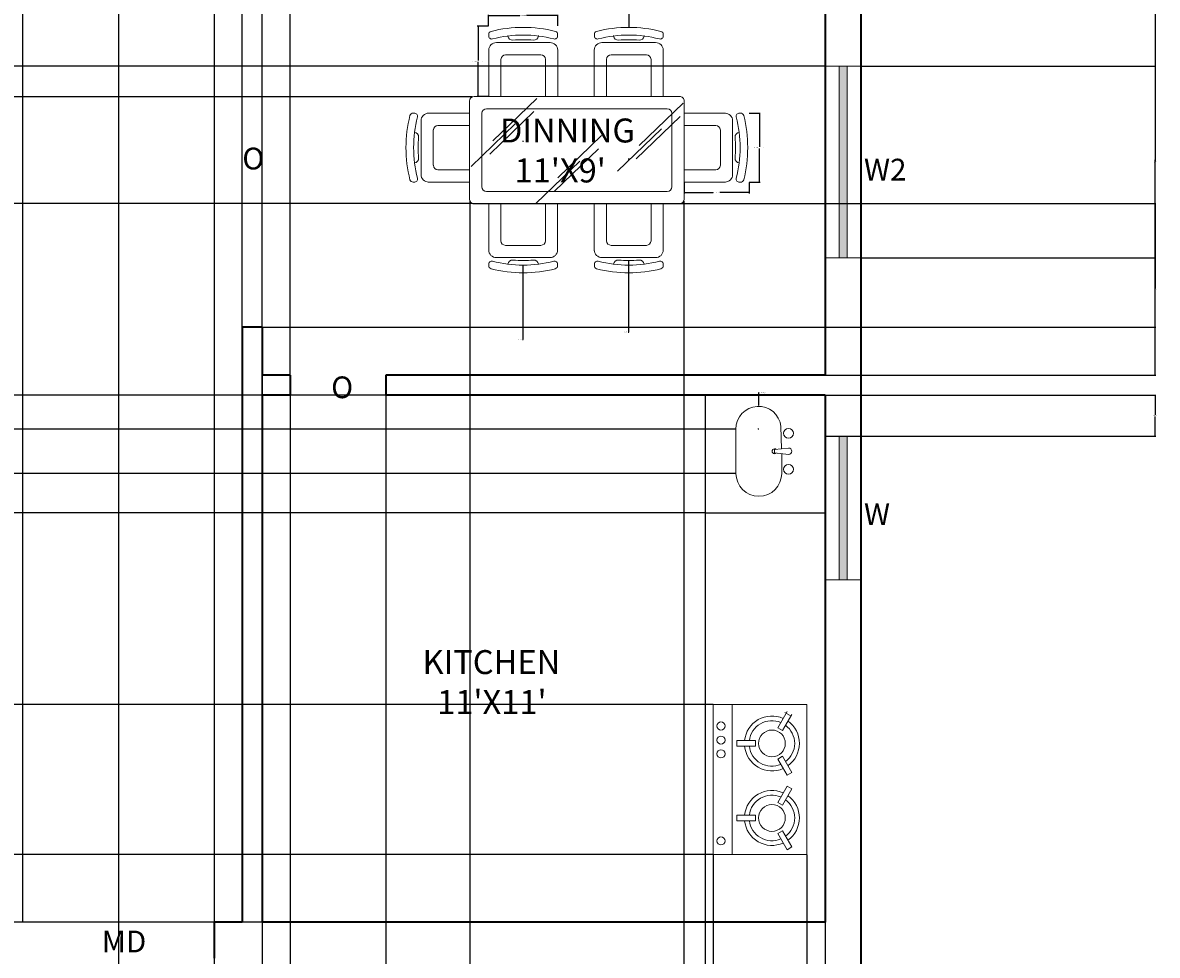
# Model space of a CAD drawing. Units: inches. Extents: x 320 to 1055, y -655 to 96.
# Tile 3 of 4: x 771 to 1055, y -389 to -155. Entities that reach past the tile are written whole.
import ezdxf

# ---------------------------------------------------------------- set-up
doc = ezdxf.new("R2010")
doc.units = ezdxf.units.IN
doc.header["$MEASUREMENT"] = 0
for name, color, linetype, lineweight in [('A-ANNO-DIMS', 2, 'Continuous', 18), ('A-ANNO-IDEN', 1, 'Continuous', 18), ('A-AREA-IDEN', 8, 'Continuous', 18), ('A-EQPM', 50, 'Continuous', 18), ('A-FLOR-CASE', 50, 'Continuous', 25), ('A-FLOR-FIXT', 50, 'Continuous', 18), ('A-GLAZ-PATT', 5, 'Continuous', 13), ('wall', 1, 'Continuous', 35), ('win', 5, 'Continuous', 18)]:
    doc.layers.add(name, color=color, linetype=linetype, lineweight=lineweight)
doc.layers.add('furniture', color=50, linetype='Continuous', lineweight=18, transparency=0.8)
doc.styles.get("Standard").update_dxf_attribs({"font": 'arial.ttf'})
doc.dimstyles.get("Standard").update_dxf_attribs({"dimtxt": 0.18, "dimasz": 0.18, "dimexe": 0.18, "dimexo": 0.0625, "dimgap": 0.09, "dimtad": 0, "dimtih": 1, "dimtoh": 1, "dimdec": 1, "dimzin": 0, "dimdsep": 46, "dimlunit": 4, "dimtxsty": 'Standard', "dimcen": 0.09, "dimadec": 0, "dimazin": 0, "dimtfac": 1, "dimtdec": 1, "dimtofl": 0, "dimtmove": 0, "dimatfit": 3, "dimfxl": 1, "dimtolj": 1, "dimtzin": 0, "dimarcsym": 0})

# ---------------------------------------------------------------- blocks, each defined once
blk = doc.blocks.new('CHAIR-DINING-SIDE')
for p, q in [((4.8, 15.13), (4.8, 15.25)), ((12.47, 15.13), (12.47, 15.25)), ((0, 11.76), (0, 11.36)), ((0, 11.58), (0, 0)), ((15.35, 13.5), (1.92, 13.5)), ((17.27, 11.36), (17.27, 11.76)), ((17.27, 0), (17.27, 11.58)), ((3.07, 9.28), (3.07, 0)), ((13.05, 10.43), (4.22, 10.43)), ((14.2, 0), (14.2, 9.28))]:
    blk.add_line(p, q)
for centre, radius, start, end in [((8.63, -15.67), 32.96, 75.853, 104.147), ((0.77, 15.54), 0.768, 104.147, 185.9216), ((-1.14, 15.34), 1.15, 354.0784, 5.9216), ((0.77, 15.15), 0.768, 174.0784, 284.3214), ((8.63, -15.67), 31.04, 75.6786, 104.3214), ((5.95, 15.25), 1.15, 186.0281, 274.9654), ((8.63, -15.67), 29.89, 85.0346, 94.9654), ((11.32, 15.25), 1.15, 265.0346, 353.9719), ((16.5, 15.15), 0.768, 255.6786, 5.9216), ((16.5, 15.54), 0.768, 354.0784, 75.853), ((18.41, 15.34), 1.15, 174.0784, 185.9216), ((1.92, 11.58), 1.92, 90, 180), ((15.35, 11.58), 1.92, 0, 90), ((4.22, 9.28), 1.15, 90, 180), ((13.05, 9.28), 1.15, 0, 90)]:
    blk.add_arc(centre, radius, start, end)
blk = doc.blocks.new('CHAIR-DINING-END')
for p, q in [((5.53, 17.27), (5.92, 17.27)), ((5.7, 17.27), (15.95, 17.27)), ((3.78, 1.92), (3.78, 15.35)), ((2.16, 12.47), (2.04, 12.47)), ((6.85, 4.22), (6.85, 13.05)), ((8.01, 14.2), (15.95, 14.2)), ((2.16, 4.8), (2.04, 4.8)), ((15.95, 3.07), (8.01, 3.07)), ((5.92, 0), (5.53, 0)), ((15.95, 0), (5.7, 0))]:
    blk.add_line(p, q)
for centre, radius, start, end in [((1.74, 16.5), 0.768, 84.0784, 165.853), ((1.94, 18.41), 1.15, 264.0784, 275.9216), ((2.14, 16.5), 0.768, 345.6786, 95.9216), ((5.7, 15.35), 1.92, 90, 180), ((32.96, 8.63), 32.96, 165.853, 194.147), ((32.96, 8.63), 31.04, 165.6786, 194.3214), ((2.04, 11.32), 1.15, 355.0346, 83.9719), ((8.01, 13.05), 1.15, 90, 180), ((32.96, 8.63), 29.89, 175.0346, 184.9654), ((2.04, 5.95), 1.15, 276.0281, 4.9654), ((8.01, 4.22), 1.15, 180, 270), ((1.74, 0.77), 0.768, 194.147, 275.9216), ((1.94, -1.14), 1.15, 84.0784, 95.9216), ((2.14, 0.77), 0.768, 264.0784, 14.3214), ((5.7, 1.92), 1.92, 180, 270)]:
    blk.add_arc(centre, radius, start, end)
blk = doc.blocks.new('WINDOW-36IN')
for p, q in [((0, 36), (9, 36)), ((3.5, 36), (3.5, 0)), ((5.5, 36), (5.5, 0)), ((0, 0), (9, 0))]:
    blk.add_line(p, q)
blk = doc.blocks.new('*D13')
at = {"layer": 'A-ANNO-DIMS', "color": 0, "lineweight": -2, "transparency": 16777216}
for p, q in [((887.51, -156.31), (884.75, -156.31)), ((884.93, -156.49), (884.93, -164.93)), ((884.93, -173.74), (884.93, -165.3)), ((887.51, -173.92), (884.75, -173.92))]:
    blk.add_line(p, q, dxfattribs=at)
at = {"layer": 'A-ANNO-DIMS', "color": 0, "transparency": 16777216}
for points in [[(884.9, -156.49), (884.96, -156.49), (884.93, -156.31)], [(884.9, -173.74), (884.96, -173.74), (884.93, -173.92)]]:
    blk.add_solid(points, dxfattribs=at)
at = {"layer": 'Defpoints', "color": 0, "transparency": 16777216}
for p in [(884.93, -156.31), (887.57, -156.31), (887.57, -173.92)]:
    blk.add_point(p, dxfattribs=at)
at = {"layer": 'A-ANNO-DIMS', "color": 0, "transparency": 16777216, "insert": (884.93, -165.12), "char_height": 0.18, "attachment_point": 5}
blk.add_mtext('\\A1;SIDE CHAIR 1\'-5 1/2" TYP.', dxfattribs=at)
blk = doc.blocks.new('*D14')
at = {"layer": 'A-ANNO-DIMS', "color": 0, "lineweight": -2, "transparency": 16777216}
for p, q in [((887.57, -156.24), (887.57, -153.48)), ((904.91, -156.24), (904.91, -153.48)), ((887.75, -153.66), (895.4, -153.66)), ((904.73, -153.66), (897.08, -153.66))]:
    blk.add_line(p, q, dxfattribs=at)
at = {"layer": 'A-ANNO-DIMS', "color": 0, "transparency": 16777216}
for points in [[(887.75, -153.63), (887.75, -153.69), (887.57, -153.66)], [(904.73, -153.63), (904.73, -153.69), (904.91, -153.66)]]:
    blk.add_solid(points, dxfattribs=at)
at = {"layer": 'Defpoints', "color": 0, "transparency": 16777216}
for p in [(887.57, -156.31), (904.91, -153.66), (904.91, -156.31)]:
    blk.add_point(p, dxfattribs=at)
at = {"layer": 'A-ANNO-DIMS', "color": 0, "transparency": 16777216, "insert": (896.24, -153.66), "char_height": 0.18, "attachment_point": 5}
blk.add_mtext('\\A1;1\'-5 1/2" TYP.', dxfattribs=at)
blk = doc.blocks.new('*D15')
at = {"layer": 'A-ANNO-DIMS', "color": 0, "lineweight": -2, "transparency": 16777216}
for p, q in [((952.89, -178.08), (955.61, -178.08)), ((955.43, -178.26), (955.43, -186.57)), ((955.43, -195.24), (955.43, -186.93)), ((952.89, -195.42), (955.61, -195.42))]:
    blk.add_line(p, q, dxfattribs=at)
at = {"layer": 'A-ANNO-DIMS', "color": 0, "transparency": 16777216}
for points in [[(955.4, -178.26), (955.46, -178.26), (955.43, -178.08)], [(955.4, -195.24), (955.46, -195.24), (955.43, -195.42)]]:
    blk.add_solid(points, dxfattribs=at)
at = {"layer": 'Defpoints', "color": 0, "transparency": 16777216}
for p in [(952.83, -178.08), (952.83, -195.42), (955.43, -195.42)]:
    blk.add_point(p, dxfattribs=at)
at = {"layer": 'A-ANNO-DIMS', "color": 0, "transparency": 16777216, "insert": (955.43, -186.75), "char_height": 0.18, "attachment_point": 5}
blk.add_mtext('\\A1;END CHAIR 1\'-5 1/2" TYP.', dxfattribs=at)
blk = doc.blocks.new('*D16')
at = {"layer": 'A-ANNO-DIMS', "color": 0, "lineweight": -2, "transparency": 16777216}
for p, q in [((936.55, -195.48), (936.55, -198.2)), ((952.83, -195.48), (952.83, -198.2)), ((936.73, -198.02), (943.85, -198.02)), ((952.65, -198.02), (945.53, -198.02))]:
    blk.add_line(p, q, dxfattribs=at)
at = {"layer": 'A-ANNO-DIMS', "color": 0, "transparency": 16777216}
for points in [[(936.73, -197.99), (936.73, -198.05), (936.55, -198.02)], [(952.65, -197.99), (952.65, -198.05), (952.83, -198.02)]]:
    blk.add_solid(points, dxfattribs=at)
at = {"layer": 'Defpoints', "color": 0, "transparency": 16777216}
for p in [(936.55, -195.42), (952.83, -195.42), (936.55, -198.02)]:
    blk.add_point(p, dxfattribs=at)
at = {"layer": 'A-ANNO-DIMS', "color": 0, "transparency": 16777216, "insert": (944.69, -198.02), "char_height": 0.18, "attachment_point": 5}
blk.add_mtext('\\A1;1\'-4 1/2" TYP.', dxfattribs=at)
blk = doc.blocks.new('*D23')
at = {"layer": 'A-ANNO-DIMS', "color": 0, "lineweight": -2, "transparency": 16777216}
for p, q in [((794.86, -80.8), (794.86, -655.29)), ((818.86, -80.8), (818.86, -655.29)), ((795.04, -655.11), (806.53, -655.11)), ((818.68, -655.11), (807.19, -655.11))]:
    blk.add_line(p, q, dxfattribs=at)
at = {"layer": 'A-ANNO-DIMS', "color": 0, "transparency": 16777216}
for points in [[(795.04, -655.08), (795.04, -655.14), (794.86, -655.11)], [(818.68, -655.08), (818.68, -655.14), (818.86, -655.11)]]:
    blk.add_solid(points, dxfattribs=at)
at = {"layer": 'Defpoints', "color": 0, "transparency": 16777216}
for p in [(794.86, -80.74), (818.86, -80.74), (818.86, -655.11)]:
    blk.add_point(p, dxfattribs=at)
at = {"layer": 'A-ANNO-DIMS', "color": 0, "transparency": 16777216, "insert": (806.86, -655.11), "char_height": 0.18, "attachment_point": 5}
blk.add_mtext('\\A1;2\'-0"', dxfattribs=at)
blk = doc.blocks.new('*D24')
at = {"layer": 'A-ANNO-DIMS', "color": 0, "lineweight": -2, "transparency": 16777216}
for p, q in [((980.92, -166.36), (1054.75, -166.36)), ((1054.57, -166.54), (1054.57, -190.18)), ((1054.57, -214.18), (1054.57, -190.54)), ((980.92, -214.36), (1054.75, -214.36))]:
    blk.add_line(p, q, dxfattribs=at)
at = {"layer": 'A-ANNO-DIMS', "color": 0, "transparency": 16777216}
for points in [[(1054.54, -166.54), (1054.6, -166.54), (1054.57, -166.36)], [(1054.54, -214.18), (1054.6, -214.18), (1054.57, -214.36)]]:
    blk.add_solid(points, dxfattribs=at)
at = {"layer": 'Defpoints', "color": 0, "transparency": 16777216}
for p in [(980.86, -166.36), (1054.57, -166.36), (980.86, -214.36)]:
    blk.add_point(p, dxfattribs=at)
at = {"layer": 'A-ANNO-DIMS', "color": 0, "transparency": 16777216, "insert": (1054.57, -190.36), "char_height": 0.18, "attachment_point": 5}
blk.add_mtext('\\A1;4\'-0"', dxfattribs=at)
blk = doc.blocks.new('*D25')
at = {"layer": 'A-ANNO-DIMS', "color": 0, "lineweight": -2, "transparency": 16777216}
for p, q in [((941.86, -380.8), (941.86, -655.29)), ((971.86, -380.8), (971.86, -655.29)), ((942.04, -655.11), (956.53, -655.11)), ((971.68, -655.11), (957.19, -655.11))]:
    blk.add_line(p, q, dxfattribs=at)
at = {"layer": 'A-ANNO-DIMS', "color": 0, "transparency": 16777216}
for points in [[(942.04, -655.08), (942.04, -655.14), (941.86, -655.11)], [(971.68, -655.08), (971.68, -655.14), (971.86, -655.11)]]:
    blk.add_solid(points, dxfattribs=at)
at = {"layer": 'Defpoints', "color": 0, "transparency": 16777216}
for p in [(941.86, -380.74), (971.86, -380.74), (941.86, -655.11)]:
    blk.add_point(p, dxfattribs=at)
at = {"layer": 'A-ANNO-DIMS', "color": 0, "transparency": 16777216, "insert": (956.86, -655.11), "char_height": 0.18, "attachment_point": 5}
blk.add_mtext('\\A1;2\'-6"', dxfattribs=at)
blk = doc.blocks.new('*D26')
at = {"layer": 'A-ANNO-DIMS', "color": 0, "lineweight": -2, "transparency": 16777216}
for p, q in [((941.8, -248.74), (320.04, -248.74)), ((320.22, -248.92), (320.22, -263.27)), ((320.22, -278), (320.22, -263.64)), ((941.8, -278.18), (320.04, -278.18))]:
    blk.add_line(p, q, dxfattribs=at)
at = {"layer": 'A-ANNO-DIMS', "color": 0, "transparency": 16777216}
for points in [[(320.19, -248.92), (320.25, -248.92), (320.22, -248.74)], [(320.19, -278), (320.25, -278), (320.22, -278.18)]]:
    blk.add_solid(points, dxfattribs=at)
at = {"layer": 'Defpoints', "color": 0, "transparency": 16777216}
for p in [(941.86, -248.74), (320.22, -278.18), (941.86, -278.18)]:
    blk.add_point(p, dxfattribs=at)
at = {"layer": 'A-ANNO-DIMS', "color": 0, "transparency": 16777216, "insert": (320.22, -263.46), "char_height": 0.18, "attachment_point": 5}
blk.add_mtext('\\A1;2\'-5 1/2"', dxfattribs=at)
blk = doc.blocks.new('*D27')
at = {"layer": 'A-ANNO-DIMS', "color": 0, "lineweight": -2, "transparency": 16777216}
for p, q in [((943.8, -326.24), (320.04, -326.24)), ((320.22, -326.42), (320.22, -344.83)), ((320.22, -363.61), (320.22, -345.2)), ((943.8, -363.79), (320.04, -363.79))]:
    blk.add_line(p, q, dxfattribs=at)
at = {"layer": 'A-ANNO-DIMS', "color": 0, "transparency": 16777216}
for points in [[(320.19, -326.42), (320.25, -326.42), (320.22, -326.24)], [(320.19, -363.61), (320.25, -363.61), (320.22, -363.79)]]:
    blk.add_solid(points, dxfattribs=at)
at = {"layer": 'Defpoints', "color": 0, "transparency": 16777216}
for p in [(943.86, -326.24), (320.22, -363.79), (943.86, -363.79)]:
    blk.add_point(p, dxfattribs=at)
at = {"layer": 'A-ANNO-DIMS', "color": 0, "transparency": 16777216, "insert": (320.22, -345.02), "char_height": 0.18, "attachment_point": 5}
blk.add_mtext('\\A1;3\'-1 1/2"', dxfattribs=at)
blk = doc.blocks.new('*D28')
at = {"layer": 'A-ANNO-DIMS', "color": 0, "lineweight": -2, "transparency": 16777216}
for p, q in [((943.86, -363.86), (943.86, -655.29)), ((967.33, -363.86), (967.33, -655.29)), ((944.04, -655.11), (955, -655.11)), ((967.15, -655.11), (956.2, -655.11))]:
    blk.add_line(p, q, dxfattribs=at)
at = {"layer": 'A-ANNO-DIMS', "color": 0, "transparency": 16777216}
for points in [[(944.04, -655.08), (944.04, -655.14), (943.86, -655.11)], [(967.15, -655.08), (967.15, -655.14), (967.33, -655.11)]]:
    blk.add_solid(points, dxfattribs=at)
at = {"layer": 'Defpoints', "color": 0, "transparency": 16777216}
for p in [(943.86, -363.79), (967.33, -363.79), (967.33, -655.11)]:
    blk.add_point(p, dxfattribs=at)
at = {"layer": 'A-ANNO-DIMS', "color": 0, "transparency": 16777216, "insert": (955.6, -655.11), "char_height": 0.18, "attachment_point": 5}
blk.add_mtext('\\A1;1\'-11 1/2"', dxfattribs=at)
blk = doc.blocks.new('*D29')
at = {"layer": 'A-ANNO-DIMS', "color": 0, "lineweight": -2, "transparency": 16777216}
for p, q in [((830.92, -147.74), (1054.75, -147.74)), ((1054.57, -147.92), (1054.57, -189.55)), ((1054.57, -231.56), (1054.57, -189.92)), ((830.92, -231.74), (1054.75, -231.74))]:
    blk.add_line(p, q, dxfattribs=at)
at = {"layer": 'A-ANNO-DIMS', "color": 0, "transparency": 16777216}
for points in [[(1054.54, -147.92), (1054.6, -147.92), (1054.57, -147.74)], [(1054.54, -231.56), (1054.6, -231.56), (1054.57, -231.74)]]:
    blk.add_solid(points, dxfattribs=at)
at = {"layer": 'Defpoints', "color": 0, "transparency": 16777216}
for p in [(830.86, -147.74), (830.86, -231.74), (1054.57, -231.74)]:
    blk.add_point(p, dxfattribs=at)
at = {"layer": 'A-ANNO-DIMS', "color": 0, "transparency": 16777216, "insert": (1054.57, -189.74), "char_height": 0.18, "attachment_point": 5}
blk.add_mtext('\\A1;7\'-0"', dxfattribs=at)
blk = doc.blocks.new('*D30')
at = {"layer": 'A-ANNO-DIMS', "color": 0, "lineweight": -2, "transparency": 16777216}
for p, q in [((837.86, -248.8), (837.86, -655.29)), ((861.86, -248.8), (861.86, -655.29)), ((838.04, -655.11), (849.53, -655.11)), ((861.68, -655.11), (850.19, -655.11))]:
    blk.add_line(p, q, dxfattribs=at)
at = {"layer": 'A-ANNO-DIMS', "color": 0, "transparency": 16777216}
for points in [[(838.04, -655.08), (838.04, -655.14), (837.86, -655.11)], [(861.68, -655.08), (861.68, -655.14), (861.86, -655.11)]]:
    blk.add_solid(points, dxfattribs=at)
at = {"layer": 'Defpoints', "color": 0, "transparency": 16777216}
for p in [(837.86, -248.74), (861.86, -248.74), (861.86, -655.11)]:
    blk.add_point(p, dxfattribs=at)
at = {"layer": 'A-ANNO-DIMS', "color": 0, "transparency": 16777216, "insert": (849.86, -655.11), "char_height": 0.18, "attachment_point": 5}
blk.add_mtext('\\A1;2\'-0"', dxfattribs=at)
blk = doc.blocks.new('*D31')
at = {"layer": 'A-ANNO-DIMS', "color": 0, "lineweight": -2, "transparency": 16777216}
for p, q in [((882.91, -200.15), (882.91, -655.29)), ((936.46, -200.15), (936.46, -655.29)), ((883.09, -655.11), (909.14, -655.11)), ((936.28, -655.11), (910.23, -655.11))]:
    blk.add_line(p, q, dxfattribs=at)
at = {"layer": 'A-ANNO-DIMS', "color": 0, "transparency": 16777216}
for points in [[(883.09, -655.08), (883.09, -655.14), (882.91, -655.11)], [(936.28, -655.08), (936.28, -655.14), (936.46, -655.11)]]:
    blk.add_solid(points, dxfattribs=at)
at = {"layer": 'Defpoints', "color": 0, "transparency": 16777216}
for p in [(882.91, -200.08), (936.46, -200.08), (936.46, -655.11)]:
    blk.add_point(p, dxfattribs=at)
at = {"layer": 'A-ANNO-DIMS', "color": 0, "transparency": 16777216, "insert": (909.68, -655.11), "char_height": 0.18, "attachment_point": 5}
blk.add_mtext('\\A1;4\'-5 1/2"', dxfattribs=at)
blk = doc.blocks.new('*D32')
at = {"layer": 'A-ANNO-DIMS', "color": 0, "lineweight": -2, "transparency": 16777216}
for p, q in [((883.46, -174.02), (320.04, -174.02)), ((320.22, -174.2), (320.22, -187.17)), ((320.22, -200.52), (320.22, -187.54)), ((883.46, -200.7), (320.04, -200.7))]:
    blk.add_line(p, q, dxfattribs=at)
at = {"layer": 'A-ANNO-DIMS', "color": 0, "transparency": 16777216}
for points in [[(320.19, -174.2), (320.25, -174.2), (320.22, -174.02)], [(320.19, -200.52), (320.25, -200.52), (320.22, -200.7)]]:
    blk.add_solid(points, dxfattribs=at)
at = {"layer": 'Defpoints', "color": 0, "transparency": 16777216}
for p in [(883.52, -174.02), (320.22, -200.7), (883.52, -200.7)]:
    blk.add_point(p, dxfattribs=at)
at = {"layer": 'A-ANNO-DIMS', "color": 0, "transparency": 16777216, "insert": (320.22, -187.36), "char_height": 0.18, "attachment_point": 5}
blk.add_mtext('\\A1;2\'-2 1/2"', dxfattribs=at)
blk = doc.blocks.new('*D40')
at = {"layer": 'A-ANNO-DIMS', "color": 0, "lineweight": -2, "transparency": 16777216}
for p, q in [((825.86, -380.67), (825.86, 47.57)), ((826.04, 47.39), (828.03, 47.39)), ((830.68, 47.39), (828.69, 47.39)), ((830.86, -380.67), (830.86, 47.57))]:
    blk.add_line(p, q, dxfattribs=at)
at = {"layer": 'A-ANNO-DIMS', "color": 0, "transparency": 16777216}
for points in [[(826.04, 47.42), (826.04, 47.36), (825.86, 47.39)], [(830.68, 47.42), (830.68, 47.36), (830.86, 47.39)]]:
    blk.add_solid(points, dxfattribs=at)
at = {"layer": 'Defpoints', "color": 0, "transparency": 16777216}
for p in [(830.86, 47.39), (825.86, -380.74), (830.86, -380.74)]:
    blk.add_point(p, dxfattribs=at)
at = {"layer": 'A-ANNO-DIMS', "color": 0, "transparency": 16777216, "insert": (828.36, 47.39), "char_height": 0.18, "attachment_point": 5}
blk.add_mtext('\\A1;0\'-5"', dxfattribs=at)
blk = doc.blocks.new('*D41')
at = {"layer": 'A-ANNO-DIMS', "color": 0, "lineweight": -2, "transparency": 16777216}
for p, q in [((971.8, -135.74), (320.04, -135.74)), ((320.22, -135.92), (320.22, -150.86)), ((320.22, -166.18), (320.22, -151.23)), ((971.8, -166.36), (320.04, -166.36))]:
    blk.add_line(p, q, dxfattribs=at)
at = {"layer": 'A-ANNO-DIMS', "color": 0, "transparency": 16777216}
for points in [[(320.19, -135.92), (320.25, -135.92), (320.22, -135.74)], [(320.19, -166.18), (320.25, -166.18), (320.22, -166.36)]]:
    blk.add_solid(points, dxfattribs=at)
at = {"layer": 'Defpoints', "color": 0, "transparency": 16777216}
for p in [(971.86, -135.74), (320.22, -166.36), (971.86, -166.36)]:
    blk.add_point(p, dxfattribs=at)
at = {"layer": 'A-ANNO-DIMS', "color": 0, "transparency": 16777216, "insert": (320.22, -151.05), "char_height": 0.18, "attachment_point": 5}
blk.add_mtext('\\A1;2\'-6 1/2"', dxfattribs=at)
blk = doc.blocks.new('*D42')
at = {"layer": 'A-ANNO-DIMS', "color": 0, "lineweight": -2, "transparency": 16777216}
for p, q in [((971.92, -248.74), (1054.75, -248.74)), ((1054.57, -248.92), (1054.57, -253.69)), ((1054.57, -258.82), (1054.57, -254.05)), ((971.92, -259), (1054.75, -259))]:
    blk.add_line(p, q, dxfattribs=at)
at = {"layer": 'A-ANNO-DIMS', "color": 0, "transparency": 16777216}
for points in [[(1054.54, -248.92), (1054.6, -248.92), (1054.57, -248.74)], [(1054.54, -258.82), (1054.6, -258.82), (1054.57, -259)]]:
    blk.add_solid(points, dxfattribs=at)
at = {"layer": 'Defpoints', "color": 0, "transparency": 16777216}
for p in [(971.86, -248.74), (971.86, -259), (1054.57, -259)]:
    blk.add_point(p, dxfattribs=at)
at = {"layer": 'A-ANNO-DIMS', "color": 0, "transparency": 16777216, "insert": (1054.57, -253.87), "char_height": 0.18, "attachment_point": 5}
blk.add_mtext('\\A1;0\'-10 1/2"', dxfattribs=at)
blk = doc.blocks.new('*D43')
at = {"layer": 'A-ANNO-DIMS', "color": 0, "lineweight": -2, "transparency": 16777216}
for p, q in [((943.8, -363.79), (320.04, -363.79)), ((320.22, -363.97), (320.22, -372.08)), ((320.22, -380.56), (320.22, -372.45)), ((941.8, -380.74), (320.04, -380.74))]:
    blk.add_line(p, q, dxfattribs=at)
at = {"layer": 'A-ANNO-DIMS', "color": 0, "transparency": 16777216}
for points in [[(320.19, -363.97), (320.25, -363.97), (320.22, -363.79)], [(320.19, -380.56), (320.25, -380.56), (320.22, -380.74)]]:
    blk.add_solid(points, dxfattribs=at)
at = {"layer": 'Defpoints', "color": 0, "transparency": 16777216}
for p in [(320.22, -363.79), (943.86, -363.79), (941.86, -380.74)]:
    blk.add_point(p, dxfattribs=at)
at = {"layer": 'A-ANNO-DIMS', "color": 0, "transparency": 16777216, "insert": (320.22, -372.26), "char_height": 0.18, "attachment_point": 5}
blk.add_mtext('\\A1;1\'-5"', dxfattribs=at)
blk = doc.blocks.new('*D44')
at = {"layer": 'A-ANNO-DIMS', "color": 0, "lineweight": -2, "transparency": 16777216}
for p, q in [((949.47, -257.26), (320.04, -257.26)), ((320.22, -257.44), (320.22, -262.61)), ((320.22, -268.14), (320.22, -262.97)), ((949.47, -268.32), (320.04, -268.32))]:
    blk.add_line(p, q, dxfattribs=at)
at = {"layer": 'A-ANNO-DIMS', "color": 0, "transparency": 16777216}
for points in [[(320.19, -257.44), (320.25, -257.44), (320.22, -257.26)], [(320.19, -268.14), (320.25, -268.14), (320.22, -268.32)]]:
    blk.add_solid(points, dxfattribs=at)
at = {"layer": 'Defpoints', "color": 0, "transparency": 16777216}
for p in [(949.54, -257.26), (320.22, -268.32), (949.54, -268.32)]:
    blk.add_point(p, dxfattribs=at)
at = {"layer": 'A-ANNO-DIMS', "color": 0, "transparency": 16777216, "insert": (320.22, -262.79), "char_height": 0.18, "attachment_point": 5}
blk.add_mtext('\\A1;0\'-11"', dxfattribs=at)
blk = doc.blocks.new('*D46')
at = {"layer": 'A-ANNO-DIMS', "color": 0, "lineweight": -2, "transparency": 16777216}
for p, q in [((758.05, -380.67), (758.05, 47.57)), ((758.23, 47.39), (764.13, 47.39)), ((770.68, 47.39), (764.77, 47.39)), ((770.86, -380.67), (770.86, 47.57))]:
    blk.add_line(p, q, dxfattribs=at)
at = {"layer": 'A-ANNO-DIMS', "color": 0, "transparency": 16777216}
for points in [[(758.23, 47.42), (758.23, 47.36), (758.05, 47.39)], [(770.68, 47.42), (770.68, 47.36), (770.86, 47.39)]]:
    blk.add_solid(points, dxfattribs=at)
at = {"layer": 'Defpoints', "color": 0, "transparency": 16777216}
for p in [(770.86, 47.39), (758.05, -380.74), (770.86, -380.74)]:
    blk.add_point(p, dxfattribs=at)
at = {"layer": 'A-ANNO-DIMS', "color": 0, "transparency": 16777216, "insert": (764.45, 47.39), "char_height": 0.18, "attachment_point": 5}
blk.add_mtext('\\A1;1\'-1"', dxfattribs=at)
blk = doc.blocks.new('*D51')
at = {"layer": 'A-ANNO-DIMS', "color": 0, "lineweight": -2, "transparency": 16777216}
for p, q in [((830.86, -248.67), (830.86, 47.57)), ((831.04, 47.39), (834.03, 47.39)), ((837.68, 47.39), (834.69, 47.39)), ((837.86, -248.67), (837.86, 47.57))]:
    blk.add_line(p, q, dxfattribs=at)
at = {"layer": 'A-ANNO-DIMS', "color": 0, "transparency": 16777216}
for points in [[(831.04, 47.42), (831.04, 47.36), (830.86, 47.39)], [(837.68, 47.42), (837.68, 47.36), (837.86, 47.39)]]:
    blk.add_solid(points, dxfattribs=at)
at = {"layer": 'Defpoints', "color": 0, "transparency": 16777216}
for p in [(837.86, 47.39), (830.86, -248.74), (837.86, -248.74)]:
    blk.add_point(p, dxfattribs=at)
at = {"layer": 'A-ANNO-DIMS', "color": 0, "transparency": 16777216, "insert": (834.36, 47.39), "char_height": 0.18, "attachment_point": 5}
blk.add_mtext('\\A1;0\'-7"', dxfattribs=at)
blk = doc.blocks.new('*D54')
at = {"layer": 'A-ANNO-DIMS', "color": 0, "lineweight": -2, "transparency": 16777216}
for p, q in [((882.91, -200.15), (882.91, -655.29)), ((830.86, -231.8), (830.86, -655.29)), ((831.04, -655.11), (856.55, -655.11)), ((882.73, -655.11), (857.22, -655.11))]:
    blk.add_line(p, q, dxfattribs=at)
at = {"layer": 'A-ANNO-DIMS', "color": 0, "transparency": 16777216}
for points in [[(831.04, -655.08), (831.04, -655.14), (830.86, -655.11)], [(882.73, -655.08), (882.73, -655.14), (882.91, -655.11)]]:
    blk.add_solid(points, dxfattribs=at)
at = {"layer": 'Defpoints', "color": 0, "transparency": 16777216}
for p in [(882.91, -200.08), (830.86, -231.74), (882.91, -655.11)]:
    blk.add_point(p, dxfattribs=at)
at = {"layer": 'A-ANNO-DIMS', "color": 0, "transparency": 16777216, "insert": (856.89, -655.11), "char_height": 0.18, "attachment_point": 5}
blk.add_mtext('\\A1;4\'-4"', dxfattribs=at)
blk = doc.blocks.new('*D55')
at = {"layer": 'A-ANNO-DIMS', "color": 0, "lineweight": -2, "transparency": 16777216}
for p, q in [((883.59, -200.7), (1054.75, -200.7)), ((1054.57, -200.88), (1054.57, -222.03)), ((1054.57, -243.56), (1054.57, -222.4)), ((861.92, -243.74), (1054.75, -243.74))]:
    blk.add_line(p, q, dxfattribs=at)
at = {"layer": 'A-ANNO-DIMS', "color": 0, "transparency": 16777216}
for points in [[(1054.54, -200.88), (1054.6, -200.88), (1054.57, -200.7)], [(1054.54, -243.56), (1054.6, -243.56), (1054.57, -243.74)]]:
    blk.add_solid(points, dxfattribs=at)
at = {"layer": 'Defpoints', "color": 0, "transparency": 16777216}
for p in [(883.52, -200.7), (861.86, -243.74), (1054.57, -243.74)]:
    blk.add_point(p, dxfattribs=at)
at = {"layer": 'A-ANNO-DIMS', "color": 0, "transparency": 16777216, "insert": (1054.57, -222.22), "char_height": 0.18, "attachment_point": 5}
blk.add_mtext('\\A1;3\'-7"', dxfattribs=at)
blk = doc.blocks.new('*D56')
at = {"layer": 'A-ANNO-DIMS', "color": 0, "lineweight": -2, "transparency": 16777216}
for p, q in [((830.86, -380.8), (830.86, -655.29)), ((941.86, -380.8), (941.86, -655.29)), ((831.04, -655.11), (886.03, -655.11)), ((941.68, -655.11), (886.69, -655.11))]:
    blk.add_line(p, q, dxfattribs=at)
at = {"layer": 'A-ANNO-DIMS', "color": 0, "transparency": 16777216}
for points in [[(831.04, -655.08), (831.04, -655.14), (830.86, -655.11)], [(941.68, -655.08), (941.68, -655.14), (941.86, -655.11)]]:
    blk.add_solid(points, dxfattribs=at)
at = {"layer": 'Defpoints', "color": 0, "transparency": 16777216}
for p in [(830.86, -380.74), (941.86, -380.74), (941.86, -655.11)]:
    blk.add_point(p, dxfattribs=at)
at = {"layer": 'A-ANNO-DIMS', "color": 0, "transparency": 16777216, "insert": (886.36, -655.11), "char_height": 0.18, "attachment_point": 5}
blk.add_mtext('\\A1;9\'-3"', dxfattribs=at)
blk = doc.blocks.new('*D58')
at = {"layer": 'A-ANNO-DIMS', "color": 0, "lineweight": -2, "transparency": 16777216}
for p, q in [((955.21, -248.13), (955.2, -251.34)), ((955.39, -248.13), (955.21, -248.13)), ((955.1, -257.17), (955.28, -257.17)), ((955.19, -257.26), (955.19, -257.08))]:
    blk.add_line(p, q, dxfattribs=at)
at = {"layer": 'A-ANNO-DIMS', "color": 0, "transparency": 16777216}
blk.add_solid([(955.17, -251.34), (955.23, -251.34), (955.2, -251.52)], dxfattribs=at)
at = {"layer": 'Defpoints', "color": 0, "transparency": 16777216}
for p in [(955.2, -251.52), (955.19, -257.17)]:
    blk.add_point(p, dxfattribs=at)
at = {"layer": 'A-ANNO-DIMS', "color": 0, "transparency": 16777216, "insert": (956.21, -248.13), "char_height": 0.18, "attachment_point": 5}
blk.add_mtext('\\A1;2X R0\'-5 1/2"', dxfattribs=at)
blk = doc.blocks.new('*D59')
at = {"layer": 'A-ANNO-DIMS', "color": 0, "lineweight": -2, "transparency": 16777216}
for p, q in [((922.51, -136.87), (922.69, -136.87)), ((922.69, -136.87), (922.69, -156.46)), ((922.6, -189.59), (922.78, -189.59)), ((922.69, -189.68), (922.69, -189.5))]:
    blk.add_line(p, q, dxfattribs=at)
at = {"layer": 'A-ANNO-DIMS', "color": 0, "transparency": 16777216}
blk.add_solid([(922.72, -156.46), (922.66, -156.46), (922.69, -156.64)], dxfattribs=at)
at = {"layer": 'Defpoints', "color": 0, "transparency": 16777216}
for p in [(922.69, -156.64), (922.69, -189.59)]:
    blk.add_point(p, dxfattribs=at)
at = {"layer": 'A-ANNO-DIMS', "color": 0, "transparency": 16777216, "insert": (921.9, -136.87), "char_height": 0.18, "attachment_point": 5}
blk.add_mtext('\\A1;6X R2\'-9"', dxfattribs=at)
blk = doc.blocks.new('*D60')
at = {"layer": 'A-ANNO-DIMS', "color": 0, "lineweight": -2, "transparency": 16777216}
for p, q in [((896.15, -185.12), (896.33, -185.12)), ((896.24, -185.21), (896.24, -185.03)), ((896.24, -234.78), (896.24, -216.33)), ((896.06, -234.78), (896.24, -234.78))]:
    blk.add_line(p, q, dxfattribs=at)
at = {"layer": 'A-ANNO-DIMS', "color": 0, "transparency": 16777216}
blk.add_solid([(896.21, -216.33), (896.27, -216.33), (896.24, -216.15)], dxfattribs=at)
at = {"layer": 'Defpoints', "color": 0, "transparency": 16777216}
for p in [(896.24, -185.12), (896.24, -216.15)]:
    blk.add_point(p, dxfattribs=at)
at = {"layer": 'A-ANNO-DIMS', "color": 0, "transparency": 16777216, "insert": (895.45, -234.78), "char_height": 0.18, "attachment_point": 5}
blk.add_mtext('\\A1;6X R2\'-7"', dxfattribs=at)
blk = doc.blocks.new('*D61')
at = {"layer": 'A-ANNO-DIMS', "color": 0, "lineweight": -2, "transparency": 16777216}
for p, q in [((922.6, -185.12), (922.78, -185.12)), ((922.69, -185.21), (922.69, -185.03)), ((922.69, -232.93), (922.69, -215.18)), ((922.51, -232.93), (922.69, -232.93))]:
    blk.add_line(p, q, dxfattribs=at)
at = {"layer": 'A-ANNO-DIMS', "color": 0, "transparency": 16777216}
blk.add_solid([(922.66, -215.18), (922.72, -215.18), (922.69, -215)], dxfattribs=at)
at = {"layer": 'Defpoints', "color": 0, "transparency": 16777216}
for p in [(922.69, -185.12), (922.69, -215)]:
    blk.add_point(p, dxfattribs=at)
at = {"layer": 'A-ANNO-DIMS', "color": 0, "transparency": 16777216, "insert": (921.9, -232.93), "char_height": 0.18, "attachment_point": 5}
blk.add_mtext('\\A1;6X R2\'-6"', dxfattribs=at)

msp = doc.modelspace()

# ---------------------------------------------------------------- hatches: boundary and pattern name
at = {"layer": 'A-GLAZ-PATT'}
h = msp.add_hatch(color=256, dxfattribs=at)
h.dxf.hatch_style = 1
h.paths.add_polyline_path([(977.36, -166.36), (975.36, -166.36), (975.36, -214.36), (977.36, -214.36)])
h.paths.add_polyline_path([(977.36, -85.01), (975.36, -85.01), (975.36, -121.01), (977.36, -121.01)])
h.paths.add_polyline_path([(818.66, 6.76), (794.66, 6.76), (794.66, 4.76), (818.66, 4.76)])
h.paths.add_polyline_path([(689.3, 6.76), (665.3, 6.76), (665.3, 4.76), (689.3, 4.76)])
h.paths.add_polyline_path([(458.36, -10.79), (456.36, -10.79), (456.36, -46.79), (458.36, -46.79)])
h.paths.add_polyline_path([(458.36, -214.05), (456.36, -214.05), (456.36, -238.05), (458.36, -238.05)])
h.paths.add_polyline_path([(458.36, -257.01), (456.36, -257.01), (456.36, -293.01), (458.36, -293.01)])
h.paths.add_polyline_path([(977.36, -259), (975.36, -259), (975.36, -295), (977.36, -295)])
h.paths.add_polyline_path([(758.05, -384.24), (698.05, -384.24), (698.05, -386.24), (758.05, -386.24)])

# ---------------------------------------------------------------- linework, layer by layer
at = {"layer": 'A-EQPM'}
for p, q in [((943.86, -363.79), (943.86, -326.24)), ((943.86, -326.24), (967.33, -326.24)), ((948.56, -363.79), (948.56, -326.24)), ((967.33, -363.79), (967.33, -326.24)), ((960, -332.03), (962.34, -327.98)), ((961.22, -332.74), (963.56, -328.69)), ((961.79, -328.18), (963.14, -328.96)), ((960, -332.03), (961.22, -332.74)), ((949.76, -336.65), (949.77, -335.24)), ((954.44, -335.24), (949.77, -335.24)), ((954.44, -336.65), (954.44, -335.24)), ((954.44, -336.65), (949.76, -336.65)), ((961.22, -339.15), (960, -339.86)), ((960, -339.86), (962.33, -343.91)), ((961.22, -339.15), (963.55, -343.21)), ((963.55, -343.21), (962.33, -343.91)), ((960, -350.7), (962.34, -346.65)), ((962.34, -346.65), (963.56, -347.35)), ((961.22, -351.4), (963.56, -347.35)), ((960, -350.7), (961.22, -351.4)), ((949.76, -355.31), (949.77, -353.9)), ((954.44, -353.9), (949.77, -353.9)), ((954.44, -355.31), (954.44, -353.9)), ((954.44, -355.31), (949.76, -355.31)), ((961.22, -357.82), (960, -358.52)), ((961.22, -357.82), (963.55, -361.87)), ((960, -358.52), (962.33, -362.57)), ((943.86, -363.79), (967.33, -363.79)), ((963.55, -361.87), (962.33, -362.57))]:
    msp.add_line(p, q, dxfattribs=at)
at = {"layer": 'A-EQPM', "extrusion": (0, 0, -1)}
for centre, major_axis, start_param, end_param in [((958.55, -335.95), (6.88, 0), 3.2451, 5.134376), ((945.79, -331.58), (0.72, 0.72), 2.35619449019219, 8.639379797371777), ((958.55, -335.95), (4.03, 4.03), 4.051123, 5.898002), ((958.55, -335.95), (4.03, 4.03), 6.145519, 7.992397), ((958.55, -335.95), (6.88, 0.01), -0.942584, 0.946692), ((945.79, -335.11), (0.72, 0.72), 2.35619449019219, 8.639379797371777), ((958.55, -335.95), (2.37, 2.37), 2.356194490192312, 8.639379797371898), ((945.79, -338.56), (0.72, 0.72), 2.35619449019219, 8.639379797371777), ((958.55, -335.95), (6.88, -0.01), 1.148752, 3.038029), ((958.55, -335.95), (4.03, -4.03), 0.385932, 2.23281), ((958.55, -354.61), (6.88, 0), 3.244173, 5.13345), ((958.55, -354.61), (4.03, -4.03), 2.480327, 4.327205), ((958.55, -354.61), (6.88, 0), -0.944011, 0.945266), ((958.55, -354.61), (2.37, 2.37), 2.356194490192306, 8.639379797371893), ((958.55, -354.61), (4.03, 4.03), 6.145519, 7.992397), ((958.55, -354.61), (6.88, -0.01), 1.14879, 3.038067), ((958.55, -354.61), (4.03, -4.03), 0.385932, 2.23281), ((945.79, -360.36), (0.72, 0.72), 2.35619449019219, 8.639379797371777)]:
    msp.add_ellipse(centre, major_axis=major_axis, ratio=1, start_param=start_param, end_param=end_param, dxfattribs=at)
at = {"layer": 'A-FLOR-CASE'}
for p, q in [((941.86, -248.74), (941.86, -380.74)), ((941.86, -278.18), (971.9, -278.18))]:
    msp.add_line(p, q, dxfattribs=at)
at = {"layer": 'A-FLOR-FIXT'}
for p, q in [((949.54, -257.26), (949.54, -268.32)), ((960.81, -256.54), (960.97, -262.18)), ((959.22, -262.38), (962.71, -261.97)), ((959.22, -263.26), (959.22, -262.38)), ((962.71, -263.61), (959.22, -263.2)), ((961.01, -263.41), (961.01, -268.32))]:
    msp.add_line(p, q, dxfattribs=at)
for centre in [(962.71, -258.28), (962.71, -267.3)]:
    msp.add_circle(centre, 1.23, dxfattribs=at)
for centre, radius, start, end in [((955.19, -257.17), 5.65, 6.3659, 180.8792), ((959.22, -262.79), 0.615, 48.1701, 311.8299), ((962.71, -262.79), 0.82, 270, 90), ((955.28, -268.32), 5.74, 180, 0)]:
    msp.add_arc(centre, radius, start, end, dxfattribs=at)
at = {"layer": 'furniture'}
for p, q in [((882.82, -175.08), (882.82, -199.64)), ((935.4, -173.92), (883.97, -173.92)), ((899.64, -174.42), (888.66, -185.05)), ((936.3, -175.6), (925.32, -186.24)), ((936.55, -199.64), (936.55, -175.08)), ((885.89, -178.15), (885.89, -196.57)), ((932.33, -176.99), (887.04, -176.99)), ((898.88, -177.74), (887.9, -188.37)), ((935.54, -178.92), (924.56, -189.55)), ((933.48, -196.57), (933.48, -178.15)), ((894.21, -180.82), (883.23, -191.46)), ((915.86, -183.7), (904.88, -194.34)), ((930.86, -182.01), (919.88, -192.64)), ((915.1, -187.02), (904.12, -197.65)), ((910.42, -190.11), (899.44, -200.74)), ((887.04, -197.72), (932.33, -197.72)), ((883.97, -200.79), (935.4, -200.79))]:
    msp.add_line(p, q, dxfattribs=at)
for centre, radius, start, end in [((883.97, -175.08), 1.15, 90, 180), ((935.45, -175.02), 1.1, 357.166, 92.834), ((887.04, -178.15), 1.15, 90, 180), ((932.33, -178.15), 1.15, 0, 90), ((887.04, -196.57), 1.15, 180, 270), ((932.33, -196.57), 1.15, 270, 0), ((883.97, -199.64), 1.15, 180, 270), ((935.4, -199.64), 1.15, 270, 0)]:
    msp.add_arc(centre, radius, start, end, dxfattribs=at)
at = {"layer": 'wall'}
for p, q in [((980.86, 10.26), (980.86, -517.74)), ((971.86, -135.74), (971.86, -243.74)), ((830.86, -231.74), (825.86, -231.74)), ((825.86, -231.74), (825.86, -380.74)), ((830.86, -231.74), (830.86, -243.74)), ((837.86, -243.74), (830.86, -243.74)), ((837.86, -243.74), (837.86, -248.74)), ((971.86, -243.74), (861.86, -243.74)), ((861.86, -243.74), (861.86, -248.74)), ((837.86, -248.74), (830.86, -248.74)), ((830.86, -248.74), (830.86, -380.74)), ((971.86, -248.74), (861.86, -248.74)), ((971.86, -248.74), (971.86, -380.74)), ((825.86, -380.74), (818.86, -380.74)), ((818.86, -380.74), (818.86, -389.74)), ((971.86, -380.74), (830.86, -380.74))]:
    msp.add_line(p, q, dxfattribs=at)
at = {"layer": 'win'}
for p, q in [((971.86, -166.36), (980.86, -166.36)), ((975.36, -166.36), (975.36, -214.36)), ((977.36, -166.36), (977.36, -214.36)), ((971.86, -214.36), (980.86, -214.36))]:
    msp.add_line(p, q, dxfattribs=at)

# ---------------------------------------------------------------- block references
at = {"layer": 'furniture'}
for name, p in [('CHAIR-DINING-SIDE', (887.61, -173.93)), ('CHAIR-DINING-SIDE', (914.06, -173.93)), ('CHAIR-DINING-END', (866.87, -195.38))]:
    msp.add_blockref(name, p, dxfattribs=at)
at = {"layer": 'furniture', "rotation": 180}
for name, p in [('CHAIR-DINING-END', (952.49, -178.12)), ('CHAIR-DINING-SIDE', (904.87, -200.79)), ('CHAIR-DINING-SIDE', (931.33, -200.79))]:
    msp.add_blockref(name, p, dxfattribs=at)
at = {"layer": 'win', "rotation": 180}
msp.add_blockref('WINDOW-36IN', (980.86, -259), dxfattribs=at)

# ---------------------------------------------------------------- texts
at = {"layer": 'A-ANNO-IDEN'}
for s, height, p in [('O', 5.44, (825.88, -192.2)), ('W2', 5.444, (981.62, -194.98)), ('O', 5.44, (848.14, -249.49)), ('W', 5.44, (981.62, -281.26)), ('MD', 5.444, (790.68, -388.27))]:
    msp.add_text(s, height=height, dxfattribs=at).set_placement(p)
at = {"layer": 'A-AREA-IDEN', "char_height": 6, "attachment_point": 1}
for s, width, insert in [("    DINNING\\P      11'X9'", 53.3957, (883.08, -179.46)), ("    KITCHEN\\P      11'X11'", 54.3765, (863.69, -312.58))]:
    msp.add_mtext_dynamic_manual_height_columns(s, width=width, gutter_width=1, heights=[0], dxfattribs=dict(at, insert=insert))

# ---------------------------------------------------------------- dimensions: what is measured, and where the dimension line sits
at = {"layer": 'A-ANNO-DIMS'}
for base, p1, p2, picture, middle in [((770.86, 47.39), (758.05, -380.74), (770.86, -380.74), '*D46', (764.45, 47.39)), ((830.86, 47.39), (825.86, -380.74), (830.86, -380.74), '*D40', (828.36, 47.39)), ((837.86, 47.39), (830.86, -248.74), (837.86, -248.74), '*D51', (834.36, 47.39)), ((818.86, -655.11), (794.86, -80.74), (818.86, -80.74), '*D23', (806.86, -655.11)), ((882.9112, -655.1081), (830.8589, -231.7361), (882.9112, -200.0844), '*D54', (856.885, -655.1081)), ((936.4561, -655.1081), (882.9112, -200.0844), (936.4561, -200.0844), '*D31', (909.6836, -655.1081)), ((861.86, -655.11), (837.86, -248.74), (861.86, -248.74), '*D30', (849.86, -655.11)), ((967.33, -655.11), (943.86, -363.79), (967.33, -363.79), '*D28', (955.6, -655.11)), ((941.86, -655.11), (830.86, -380.74), (941.86, -380.74), '*D56', (886.36, -655.11)), ((941.86, -655.11), (971.86, -380.74), (941.86, -380.74), '*D25', (956.86, -655.11))]:
    dim = msp.add_linear_dim(base=base, p1=p1, p2=p2, dimstyle='Standard', override={"dimdec": 1, "dimlfac": 1, "dimrnd": 0, "dimzin": 1, "dimdsep": 46, "dimlunit": 4, "dimfrac": 2}, dxfattribs=at)
    dim.commit()
    dim.dimension.update_dxf_attribs({"geometry": picture, "text_midpoint": middle})
for base, p1, p2, picture, middle in [((320.22, -166.36), (971.86, -135.74), (971.86, -166.36), '*D41', (320.22, -151.05)), ((1054.57, -231.74), (830.86, -147.74), (830.86, -231.74), '*D29', (1054.57, -189.74)), ((1054.57, -166.36), (980.86, -214.36), (980.86, -166.36), '*D24', (1054.57, -190.36)), ((320.22, -200.7), (883.52, -174.02), (883.52, -200.7), '*D32', (320.22, -187.36)), ((1054.57, -243.74), (883.52, -200.7), (861.86, -243.74), '*D55', (1054.57, -222.22)), ((320.22, -278.18), (941.86, -248.74), (941.86, -278.18), '*D26', (320.22, -263.46)), ((1054.57, -259), (971.86, -248.74), (971.86, -259), '*D42', (1054.57, -253.87)), ((320.22, -268.32), (949.54, -257.26), (949.54, -268.32), '*D44', (320.22, -262.79)), ((320.2225, -363.7938), (943.8635, -326.2397), (943.8635, -363.7938), '*D27', (320.2225, -345.0167)), ((320.2225, -363.7938), (941.8589, -380.7361), (943.8635, -363.7938), '*D43', (320.2225, -372.265))]:
    dim = msp.add_linear_dim(base=base, p1=p1, p2=p2, angle=90, dimstyle='Standard', override={"dimdec": 1, "dimlfac": 1, "dimrnd": 0, "dimzin": 1, "dimdsep": 46, "dimlunit": 4, "dimfrac": 2}, dxfattribs=at)
    dim.commit()
    dim.dimension.update_dxf_attribs({"geometry": picture, "text_midpoint": middle})
for center, mpoint, text, picture, middle in [((922.6941, -189.5943), (922.694, -156.6392), '6X <>', '*D59', (921.9047, -136.8662)), ((896.24, -185.12), (896.24, -216.15), '6X <>', '*D60', (895.45, -234.78)), ((922.69, -185.12), (922.69, -215), '6X <>', '*D61', (921.9, -232.93)), ((955.19, -257.17), (955.2, -251.52), '2X <>', '*D58', (956.21, -248.13))]:
    dim = msp.add_radius_dim(center=center, mpoint=mpoint, text=text, dimstyle='Standard', override={"dimdec": 1, "dimlfac": 1, "dimrnd": 0, "dimzin": 1, "dimdsep": 46, "dimlunit": 4, "dimfrac": 2}, dxfattribs=at)
    dim.commit()
    dim.dimension.update_dxf_attribs({"geometry": picture, "text_midpoint": middle, "dimtype": 164})
dim = msp.add_linear_dim(base=(904.91, -153.66), p1=(887.57, -156.31), p2=(904.91, -156.31), text='<> TYP.', dimstyle='Standard', override={"dimdec": 1, "dimlfac": 1, "dimrnd": 0, "dimzin": 1, "dimdsep": 46, "dimlunit": 4, "dimfrac": 2}, dxfattribs=at)
dim.commit()
dim.dimension.update_dxf_attribs({"geometry": '*D14', "text_midpoint": (896.24, -153.66)})
for base, p1, p2, angle, text, picture, middle in [((884.93, -156.31), (887.57, -173.92), (887.57, -156.31), 90, 'SIDE CHAIR <> TYP.', '*D13', (884.93, -165.12)), ((955.43, -195.42), (952.83, -178.08), (952.83, -195.42), 270, 'END CHAIR <> TYP.', '*D15', (955.43, -186.75)), ((936.55, -198.02), (952.83, -195.42), (936.55, -195.42), 180, '<> TYP.', '*D16', (944.69, -198.02))]:
    dim = msp.add_linear_dim(base=base, p1=p1, p2=p2, angle=angle, text=text, dimstyle='Standard', override={"dimdec": 1, "dimlfac": 1, "dimrnd": 0, "dimzin": 1, "dimdsep": 46, "dimlunit": 4, "dimfrac": 2}, dxfattribs=at)
    dim.commit()
    dim.dimension.update_dxf_attribs({"geometry": picture, "text_midpoint": middle})

doc.saveas('drawing.dxf')
